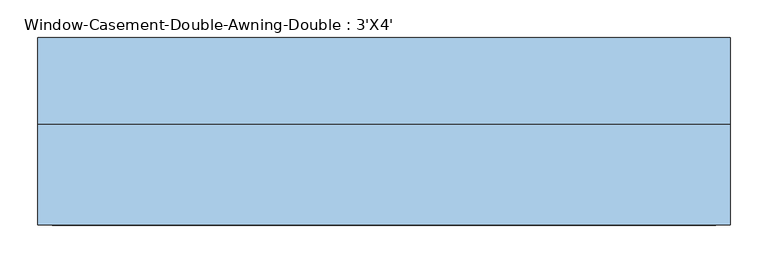
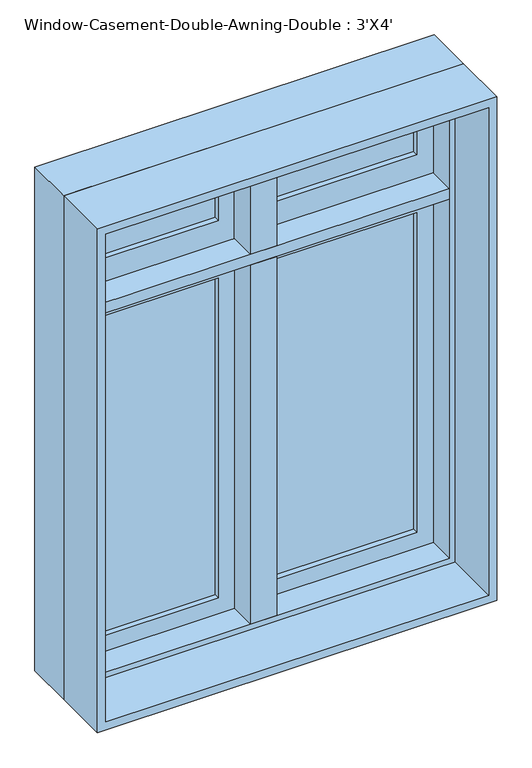
"""IFC4 building model written with IfcOpenShell, lengths in millimetres: window geometry, Window-Casement-Double-Awning-Double : 3'X4'."""

from ifc_helpers import new_model, si_unit, frame, origin, place, context, project, spatial, polyline, outline, extrude, faceted_brep, source, transform, mapped, element, save


def window_casement_double_awning_double_3_x4_7dc4ce09(model_context):
    return source(origin(), model_context, "Body", "SolidModel", [
        faceted_brep([(425.45, 82.55, 2101.85), (425.45, 19.05, 2101.85), (-425.45, 19.05, 2101.85), (-425.45, 82.55, 2101.85), (444.5, 133.35, 2120.9), (444.5, 82.55, 2120.9), (-444.5, 82.55, 2120.9), (-444.5, 133.35, 2120.9), (457.2, 19.05, 2133.6), (457.2, 133.35, 2133.6), (-457.2, 133.35, 2133.6), (-457.2, 19.05, 2133.6), (-425.45, 19.05, 946.15), (-425.45, 82.55, 946.15), (-444.5, 82.55, 927.1), (-444.5, 133.35, 927.1), (-457.2, 133.35, 914.4), (-457.2, 19.05, 914.4), (425.45, 19.05, 946.15), (425.45, 82.55, 946.15), (444.5, 82.55, 927.1), (444.5, 133.35, 927.1), (457.2, 133.35, 914.4), (457.2, 19.05, 914.4)], [[[0, 1, 2, 3]], [[4, 5, 6, 7]], [[8, 9, 10, 11]], [[3, 2, 12, 13]], [[7, 6, 14, 15]], [[11, 10, 16, 17]], [[13, 12, 18, 19]], [[15, 14, 20, 21]], [[17, 16, 22, 23]], [[11, 17, 23, 8], [1, 18, 12, 2]], [[19, 18, 1, 0]], [[5, 20, 14, 6], [3, 13, 19, 0]], [[21, 20, 5, 4]], [[23, 22, 9, 8]], [[9, 22, 16, 10], [7, 15, 21, 4]]]),
        extrude(outline(polyline([(2133.6, -457.2), (914.4, -457.2), (914.4, 457.2), (2133.6, 457.2), (2133.6, -457.2)]), holes=[polyline([(2114.55, 438.15), (933.45, 438.15), (933.45, -438.15), (2114.55, -438.15), (2114.55, 438.15)])]), frame((0.0, -114.3, 0.0), z_axis=(0.0, 1.0, 0.0), x_axis=(0.0, 0.0, 1.0)), (0.0, 0.0, 1.0), 133.35),
        extrude(outline(polyline([(927.1, 444.5), (1816.1, 444.5), (1816.1, 9.525), (927.1, 9.525), (927.1, 444.5)]), holes=[polyline([(984.25, 66.675), (1758.95, 66.675), (1758.95, 387.35), (984.25, 387.35), (984.25, 66.675)])]), frame((0.0, 82.55, 0.0), z_axis=(0.0, 1.0, 0.0), x_axis=(0.0, 0.0, 1.0)), (0.0, 0.0, 1.0), 44.45),
        extrude(outline(polyline([(1816.1, -444.5), (927.1, -444.5), (927.1, -9.525), (1816.1, -9.525), (1816.1, -444.5)]), holes=[polyline([(1758.95, -66.675), (984.25, -66.675), (984.25, -387.35), (1758.95, -387.35), (1758.95, -66.675)])]), frame((0.0, 82.55, 0.0), z_axis=(0.0, 1.0, 0.0), x_axis=(0.0, 0.0, 1.0)), (0.0, 0.0, 1.0), 44.45),
        extrude(outline(polyline([(387.35, 114.3), (387.35, 107.95), (66.675, 107.95), (66.675, 114.3), (387.35, 114.3)])), frame((0.0, 0.0, 984.25), z_axis=(0.0, 0.0, 1.0), x_axis=(1.0, 0.0, 0.0)), (0.0, 0.0, 1.0), 774.7),
        extrude(outline(polyline([(66.675, 95.25), (66.675, 101.6), (387.35, 101.6), (387.35, 95.25), (66.675, 95.25)])), frame((0.0, 0.0, 984.25), z_axis=(0.0, 0.0, 1.0), x_axis=(1.0, 0.0, 0.0)), (0.0, 0.0, 1.0), 774.7),
        extrude(outline(polyline([(-66.675, 114.3), (-66.675, 107.95), (-387.35, 107.95), (-387.35, 114.3), (-66.675, 114.3)])), frame((0.0, 0.0, 984.25), z_axis=(0.0, 0.0, 1.0), x_axis=(1.0, 0.0, 0.0)), (0.0, 0.0, 1.0), 774.7),
        extrude(outline(polyline([(-387.35, 95.25), (-387.35, 101.6), (-66.675, 101.6), (-66.675, 95.25), (-387.35, 95.25)])), frame((0.0, 0.0, 984.25), z_axis=(0.0, 0.0, 1.0), x_axis=(1.0, 0.0, 0.0)), (0.0, 0.0, 1.0), 774.7),
        faceted_brep([(9.525, 133.35, 1816.1), (-9.525, 133.35, 1816.1), (-9.525, 82.55, 1816.1), (-30.1625, 82.55, 1816.1), (-30.1625, 19.05, 1816.1), (30.1625, 19.05, 1816.1), (30.1625, 82.55, 1816.1), (9.525, 82.55, 1816.1), (9.525, 133.35, 927.1), (9.525, 82.55, 927.1), (-9.525, 82.55, 927.1), (-9.525, 133.35, 927.1), (-9.525, 82.55, 946.15), (-30.1625, 82.55, 946.15), (-30.1625, 19.05, 946.15), (30.1625, 19.05, 946.15), (30.1625, 82.55, 946.15), (9.525, 82.55, 946.15)], [[[0, 1, 2, 3, 4, 5, 6, 7]], [[8, 9, 10, 11]], [[1, 0, 8, 11]], [[2, 1, 11, 10, 12]], [[3, 2, 12, 13]], [[4, 3, 13, 14]], [[5, 4, 14, 15]], [[6, 5, 15, 16]], [[7, 6, 16, 17]], [[0, 7, 17, 9, 8]], [[17, 12, 10, 9]], [[12, 17, 16, 15, 14, 13]]]),
        extrude(outline(polyline([(-66.675, 114.3), (-66.675, 107.95), (-387.35, 107.95), (-387.35, 114.3), (-66.675, 114.3)])), frame((0.0, 0.0, 1898.65), z_axis=(0.0, 0.0, 1.0), x_axis=(1.0, 0.0, 0.0)), (0.0, 0.0, 1.0), 165.1),
        extrude(outline(polyline([(-387.35, 95.25), (-387.35, 101.6), (-66.675, 101.6), (-66.675, 95.25), (-387.35, 95.25)])), frame((0.0, 0.0, 1898.65), z_axis=(0.0, 0.0, 1.0), x_axis=(1.0, 0.0, 0.0)), (0.0, 0.0, 1.0), 165.1),
        extrude(outline(polyline([(444.5, 133.35), (444.5, 82.55), (425.45, 82.55), (425.45, 19.05), (-425.45, 19.05), (-425.45, 82.55), (-444.5, 82.55), (-444.5, 133.35), (444.5, 133.35)])), frame((0.0, 0.0, 1816.1), z_axis=(0.0, 0.0, 1.0), x_axis=(1.0, 0.0, 0.0)), (0.0, 0.0, 1.0), 25.4),
        faceted_brep([(9.525, 82.55, 2120.9), (9.525, 133.35, 2120.9), (-9.525, 133.35, 2120.9), (-9.525, 82.55, 2120.9), (-9.525, 82.55, 1841.5), (-9.525, 133.35, 1841.5), (9.525, 133.35, 1841.5), (9.525, 82.55, 1841.5), (30.1625, 82.55, 1841.5), (30.1625, 19.05, 1841.5), (-30.1625, 19.05, 1841.5), (-30.1625, 82.55, 1841.5), (-30.1625, 82.55, 2101.85), (-9.525, 82.55, 2101.85), (-30.1625, 19.05, 2101.85), (30.1625, 19.05, 2101.85), (30.1625, 82.55, 2101.85), (9.525, 82.55, 2101.85)], [[[0, 1, 2, 3]], [[4, 5, 6, 7, 8, 9, 10, 11]], [[4, 11, 12, 13]], [[11, 10, 14, 12]], [[10, 9, 15, 14]], [[9, 8, 16, 15]], [[8, 7, 17, 16]], [[1, 0, 17, 7, 6]], [[2, 1, 6, 5]], [[3, 2, 5, 4, 13]], [[17, 13, 12, 14, 15, 16]], [[13, 17, 0, 3]]]),
        extrude(outline(polyline([(2120.9, 9.525), (1841.5, 9.525), (1841.5, 444.5), (2120.9, 444.5), (2120.9, 9.525)]), holes=[polyline([(2063.75, 387.35), (1898.65, 387.35), (1898.65, 66.675), (2063.75, 66.675), (2063.75, 387.35)])]), frame((0.0, 82.55, 0.0), z_axis=(0.0, 1.0, 0.0), x_axis=(0.0, 0.0, 1.0)), (0.0, 0.0, 1.0), 44.45),
        extrude(outline(polyline([(1841.5, -9.525), (2120.9, -9.525), (2120.9, -444.5), (1841.5, -444.5), (1841.5, -9.525)]), holes=[polyline([(1898.65, -387.35), (2063.75, -387.35), (2063.75, -66.675), (1898.65, -66.675), (1898.65, -387.35)])]), frame((0.0, 82.55, 0.0), z_axis=(0.0, 1.0, 0.0), x_axis=(0.0, 0.0, 1.0)), (0.0, 0.0, 1.0), 44.45),
        extrude(outline(polyline([(66.675, 114.3), (387.35, 114.3), (387.35, 107.95), (66.675, 107.95), (66.675, 114.3)])), frame((0.0, 0.0, 1898.65), z_axis=(0.0, 0.0, 1.0), x_axis=(1.0, 0.0, 0.0)), (0.0, 0.0, 1.0), 165.1),
        extrude(outline(polyline([(387.35, 95.25), (66.675, 95.25), (66.675, 101.6), (387.35, 101.6), (387.35, 95.25)])), frame((0.0, 0.0, 1898.65), z_axis=(0.0, 0.0, 1.0), x_axis=(1.0, 0.0, 0.0)), (0.0, 0.0, 1.0), 165.1),
    ])


if __name__ == "__main__":
    model = new_model("IFC4")
    model_context = context("Model", 3, world=origin())
    ifc_project = project(units=[si_unit("LENGTHUNIT", "METRE", prefix="MILLI")], contexts=[model_context])
    site = spatial("IfcSite", under=ifc_project)
    building = spatial("IfcBuilding", under=site)
    placement = place(None, origin())
    window_casement_double_awning_double_3_x4_shape = window_casement_double_awning_double_3_x4_7dc4ce09(model_context)
    element("IfcWindow", 1, ObjectType="Window-Casement-Double-Awning-Double : 3'X4'", at=placement, inside=building, context=model_context, shape_type="MappedRepresentation", body=[
        mapped(window_casement_double_awning_double_3_x4_shape, transform((0.0, 0.0, 0.0), x_axis=(1.0, 0.0, 0.0), y_axis=(0.0, 1.0, 0.0), z_axis=(0.0, 0.0, 1.0))),
    ])
    save(model, "model.ifc")

# Revit data of these elements
# Type "Window-Casement-Double-Awning-Double : 3'X4'"
#   Type Mark = "20"
#   Fire Rating = "0.5h"
#   Assembly Code = "B2020100"
#   Analytic Construction = "Double glazing - domestic"
#   Window Inset [instance default] = 0' - 0"
#   Wall Thickness [instance default] = 0' - 6"
#   Interior Wall Closure [instance default] = 0' - 2 1/4"
#   Half Width = 1' - 6"
#   Visual Light Transmittance = 0.81
#   Transom Height = 1' - 0"
#   Thermal Resistance (R) = 1.8146 (h·ft²·°F)/BTU
#   Solar Heat Gain Coefficient = 0.76
#   Rough Width = 3' - 0 1/2"
#   Rough Height = 4' - 0 1/2"
#   Open Window Height = 3' - 0"
#   Frame Extension [instance default] = 0' - 0 1/4"
#   Height = 4' - 0"
#   Heat Transfer Coefficient (U) = 0.5511 BTU/(h·ft²·°F)
#   Exterior Wall Closure [instance default] = 0' - 1 1/4"
#   Extension Jamb [instance default] = 0' - 2 1/4"
#   Default Sill Height = 3' - 0"
#   Width = 3' - 0"
#   Top Muntin Visibility = yes
#   Bottom Muntin Visibility = yes
#   Interior Trim Visibility [instance default] = yes
#   Exterior Trim Visibility [instance default] = yes
#   Extension Jamb Visibility [instance default] = yes
#   Interior Trim Material = Wood - Stained
#   Muntin Pattern = Muntin Pattern_2x2 : Muntin Pattern_2x2
#   Interior Trim = Trim-Window-Interior-Flat : Picture Frame
#   Interior Frame Material = Wood - Stained
#   Glass Panel Material = Glass
#   Exterior Trim Material = Clad - White
#   Exterior Trim = Trim-Window-Exterior-Flat : with Sill
#   Exterior Frame Material = Clad - White
#   Wall Closure = (empty or 0)
# Element 1 (IfcWindow, "Window-Casement-Double-Awning-Double : 3'X4'")
#   Wall Thickness = 0' - 9"
#   Extension Jamb = 0' - 5 1/4"
#   Materials on its faces: "Wood - Stained", "Glass", "Clad - White"
# Materials
#   "Wood - Stained": class "Wood", colour RGB 224 178 126, transparency 0, Cost = 0
#   "Glass": class "Glass", colour RGB 0 128 192, transparency 0.75, Description = "Soda Lime Glass", Cost = 0
#   "Clad - White": class "Wood", colour RGB 242 242 238, transparency 0, Cost = 0
